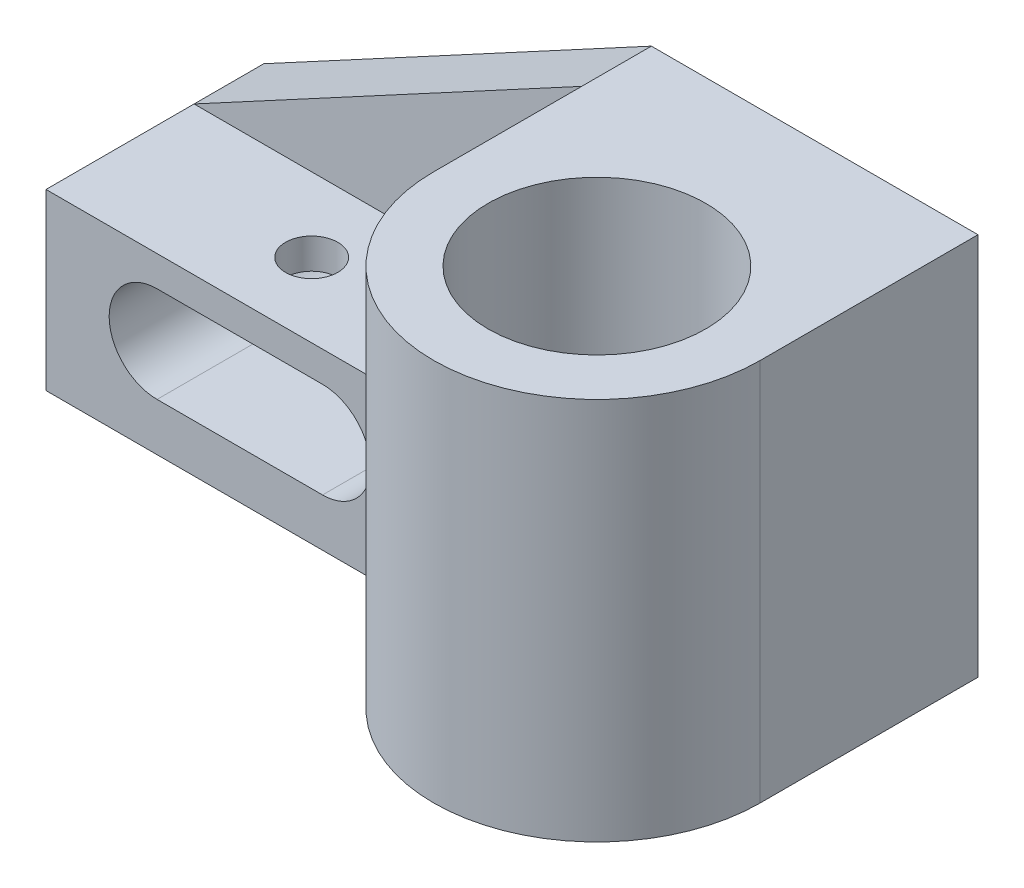
ISO-10303-21;
HEADER;
FILE_DESCRIPTION(('STEP AP214'),'2;1');
FILE_NAME('part.step','',(''),(''),'','','');
FILE_SCHEMA(('AUTOMOTIVE_DESIGN { 1 0 10303 214 1 1 1 1 }'));
ENDSEC;
DATA;
#1=APPLICATION_CONTEXT('core data for automotive mechanical design processes');
#2=APPLICATION_PROTOCOL_DEFINITION('international standard','automotive_design',2000,#1);
#3=PRODUCT_CONTEXT('',#1,'mechanical');
#4=PRODUCT('Part','Part','',(#3));
#5=PRODUCT_RELATED_PRODUCT_CATEGORY('part','',(#4));
#6=PRODUCT_DEFINITION_FORMATION('','',#4);
#7=PRODUCT_DEFINITION_CONTEXT('part definition',#1,'design');
#8=PRODUCT_DEFINITION('design','',#6,#7);
#9=PRODUCT_DEFINITION_SHAPE('','',#8);
#10=(LENGTH_UNIT() NAMED_UNIT(*) SI_UNIT(.MILLI.,.METRE.));
#11=(NAMED_UNIT(*) PLANE_ANGLE_UNIT() SI_UNIT($,.RADIAN.));
#12=(NAMED_UNIT(*) SI_UNIT($,.STERADIAN.) SOLID_ANGLE_UNIT());
#13=UNCERTAINTY_MEASURE_WITH_UNIT(LENGTH_MEASURE(1.E-05),#10,'distance_accuracy_value','');
#14=(GEOMETRIC_REPRESENTATION_CONTEXT(3) GLOBAL_UNCERTAINTY_ASSIGNED_CONTEXT((#13)) GLOBAL_UNIT_ASSIGNED_CONTEXT((#10,
#11,#12)) REPRESENTATION_CONTEXT('',''));
#15=CARTESIAN_POINT('',(0.,0.,0.));
#16=DIRECTION('',(0.,0.,1.));
#17=DIRECTION('',(1.,0.,0.));
#18=AXIS2_PLACEMENT_3D('',#15,#16,#17);
#19=CARTESIAN_POINT('',(89.,44.,50.));
#20=DIRECTION('',(1.,0.,0.));
#21=DIRECTION('',(0.,0.,-1.));
#22=AXIS2_PLACEMENT_3D('',#19,#20,#21);
#23=PLANE('',#22);
#24=DIRECTION('',(0.,0.,1.));
#25=VECTOR('',#24,1.);
#26=CARTESIAN_POINT('',(89.,48.,50.));
#27=LINE('',#26,#25);
#28=CARTESIAN_POINT('',(89.,48.,16.));
#29=VERTEX_POINT('',#28);
#30=CARTESIAN_POINT('',(89.,48.,50.));
#31=VERTEX_POINT('',#30);
#32=EDGE_CURVE('E179',#29,#31,#27,.T.);
#33=ORIENTED_EDGE('',*,*,#32,.F.);
#34=DIRECTION('',(0.,-1.,0.));
#35=VECTOR('',#34,1.);
#36=CARTESIAN_POINT('',(89.,44.,16.));
#37=LINE('',#36,#35);
#38=CARTESIAN_POINT('',(89.,0.,16.));
#39=VERTEX_POINT('',#38);
#40=EDGE_CURVE('E197',#29,#39,#37,.T.);
#41=ORIENTED_EDGE('',*,*,#40,.T.);
#42=DIRECTION('',(0.,0.,1.));
#43=VECTOR('',#42,1.);
#44=CARTESIAN_POINT('',(89.,0.,50.));
#45=LINE('',#44,#43);
#46=CARTESIAN_POINT('',(89.,0.,50.));
#47=VERTEX_POINT('',#46);
#48=EDGE_CURVE('E207',#39,#47,#45,.T.);
#49=ORIENTED_EDGE('',*,*,#48,.T.);
#50=DIRECTION('',(0.,-1.,0.));
#51=VECTOR('',#50,1.);
#52=CARTESIAN_POINT('',(89.,44.,50.));
#53=LINE('',#52,#51);
#54=EDGE_CURVE('E206',#31,#47,#53,.T.);
#55=ORIENTED_EDGE('',*,*,#54,.F.);
#56=EDGE_LOOP('',(#33,#41,#49,#55));
#57=FACE_BOUND('',#56,.T.);
#58=ADVANCED_FACE('F44',(#57),#23,.F.);
#59=CARTESIAN_POINT('',(0.,0.,0.));
#60=DIRECTION('',(0.,0.,1.));
#61=DIRECTION('',(1.,0.,0.));
#62=AXIS2_PLACEMENT_3D('',#59,#60,#61);
#63=PLANE('',#62);
#64=CARTESIAN_POINT('',(25.5,-18.,0.));
#65=DIRECTION('',(0.,0.,1.));
#66=DIRECTION('',(1.,0.,0.));
#67=AXIS2_PLACEMENT_3D('',#64,#65,#66);
#68=CIRCLE('',#67,11.);
#69=CARTESIAN_POINT('',(25.5,-7.,0.));
#70=VERTEX_POINT('',#69);
#71=CARTESIAN_POINT('',(25.5,-29.,0.));
#72=VERTEX_POINT('',#71);
#73=EDGE_CURVE('E138',#70,#72,#68,.T.);
#74=ORIENTED_EDGE('',*,*,#73,.T.);
#75=DIRECTION('',(1.,0.,0.));
#76=VECTOR('',#75,1.);
#77=CARTESIAN_POINT('',(0.,-29.,0.));
#78=LINE('',#77,#76);
#79=CARTESIAN_POINT('',(63.5,-29.,0.));
#80=VERTEX_POINT('',#79);
#81=EDGE_CURVE('E134',#72,#80,#78,.T.);
#82=ORIENTED_EDGE('',*,*,#81,.T.);
#83=CARTESIAN_POINT('',(63.5,-18.,0.));
#84=DIRECTION('',(0.,0.,1.));
#85=DIRECTION('',(1.,0.,0.));
#86=AXIS2_PLACEMENT_3D('',#83,#84,#85);
#87=CIRCLE('',#86,11.);
#88=CARTESIAN_POINT('',(63.5,-7.00000000000001,0.));
#89=VERTEX_POINT('',#88);
#90=EDGE_CURVE('E142',#80,#89,#87,.T.);
#91=ORIENTED_EDGE('',*,*,#90,.T.);
#92=DIRECTION('',(1.,0.,0.));
#93=VECTOR('',#92,1.);
#94=CARTESIAN_POINT('',(0.,-6.99999999999999,0.));
#95=LINE('',#94,#93);
#96=EDGE_CURVE('E143',#70,#89,#95,.T.);
#97=ORIENTED_EDGE('',*,*,#96,.F.);
#98=EDGE_LOOP('',(#74,#82,#91,#97));
#99=FACE_BOUND('',#98,.T.);
#100=DIRECTION('',(0.,1.,0.));
#101=VECTOR('',#100,1.);
#102=CARTESIAN_POINT('',(164.,-44.,0.));
#103=LINE('',#102,#101);
#104=CARTESIAN_POINT('',(164.,-40.,0.));
#105=VERTEX_POINT('',#104);
#106=CARTESIAN_POINT('',(164.,48.,0.));
#107=VERTEX_POINT('',#106);
#108=EDGE_CURVE('E211',#105,#107,#103,.T.);
#109=ORIENTED_EDGE('',*,*,#108,.F.);
#110=DIRECTION('',(1.,0.,0.));
#111=VECTOR('',#110,1.);
#112=CARTESIAN_POINT('',(0.,-40.,0.));
#113=LINE('',#112,#111);
#114=CARTESIAN_POINT('',(0.,-40.,0.));
#115=VERTEX_POINT('',#114);
#116=EDGE_CURVE('E219',#115,#105,#113,.T.);
#117=ORIENTED_EDGE('',*,*,#116,.F.);
#118=DIRECTION('',(0.,-1.,0.));
#119=VECTOR('',#118,1.);
#120=CARTESIAN_POINT('',(0.,0.,0.));
#121=LINE('',#120,#119);
#122=CARTESIAN_POINT('',(0.,0.,0.));
#123=VERTEX_POINT('',#122);
#124=EDGE_CURVE('E213',#123,#115,#121,.T.);
#125=ORIENTED_EDGE('',*,*,#124,.F.);
#126=DIRECTION('',(0.880153354052785,0.474689449376783,0.));
#127=VECTOR('',#126,1.);
#128=CARTESIAN_POINT('',(0.,0.,0.));
#129=LINE('',#128,#127);
#130=CARTESIAN_POINT('',(89.,48.,0.));
#131=VERTEX_POINT('',#130);
#132=EDGE_CURVE('E172',#123,#131,#129,.T.);
#133=ORIENTED_EDGE('',*,*,#132,.T.);
#134=DIRECTION('',(-1.,0.,0.));
#135=VECTOR('',#134,1.);
#136=CARTESIAN_POINT('',(89.,48.,0.));
#137=LINE('',#136,#135);
#138=EDGE_CURVE('E191',#107,#131,#137,.T.);
#139=ORIENTED_EDGE('',*,*,#138,.F.);
#140=EDGE_LOOP('',(#109,#117,#125,#133,#139));
#141=FACE_BOUND('',#140,.T.);
#142=ADVANCED_FACE('F146',(#99,#141),#63,.F.);
#143=CARTESIAN_POINT('',(164.,-44.,16.));
#144=DIRECTION('',(1.,0.,0.));
#145=DIRECTION('',(0.,0.,-1.));
#146=AXIS2_PLACEMENT_3D('',#143,#144,#145);
#147=PLANE('',#146);
#148=DIRECTION('',(0.,1.,0.));
#149=VECTOR('',#148,1.);
#150=CARTESIAN_POINT('',(164.,-44.,50.));
#151=LINE('',#150,#149);
#152=CARTESIAN_POINT('',(164.,-40.,50.));
#153=VERTEX_POINT('',#152);
#154=CARTESIAN_POINT('',(164.,48.,50.));
#155=VERTEX_POINT('',#154);
#156=EDGE_CURVE('E214',#153,#155,#151,.T.);
#157=ORIENTED_EDGE('',*,*,#156,.F.);
#158=DIRECTION('',(0.,0.,1.));
#159=VECTOR('',#158,1.);
#160=CARTESIAN_POINT('',(164.,-40.,50.));
#161=LINE('',#160,#159);
#162=EDGE_CURVE('E192',#105,#153,#161,.T.);
#163=ORIENTED_EDGE('',*,*,#162,.F.);
#164=ORIENTED_EDGE('',*,*,#108,.T.);
#165=DIRECTION('',(0.,0.,-1.));
#166=VECTOR('',#165,1.);
#167=CARTESIAN_POINT('',(164.,48.,0.));
#168=LINE('',#167,#166);
#169=EDGE_CURVE('E186',#155,#107,#168,.T.);
#170=ORIENTED_EDGE('',*,*,#169,.F.);
#171=EDGE_LOOP('',(#157,#163,#164,#170));
#172=FACE_BOUND('',#171,.T.);
#173=ADVANCED_FACE('F256',(#172),#147,.T.);
#174=CARTESIAN_POINT('',(126.5,-44.,50.));
#175=DIRECTION('',(0.,1.,0.));
#176=DIRECTION('',(0.,0.,1.));
#177=AXIS2_PLACEMENT_3D('',#174,#175,#176);
#178=CYLINDRICAL_SURFACE('',#177,37.5);
#179=DIRECTION('',(0.,1.,0.));
#180=VECTOR('',#179,1.);
#181=CARTESIAN_POINT('',(89.,-40.,50.));
#182=LINE('',#181,#180);
#183=CARTESIAN_POINT('',(89.,-40.,50.));
#184=VERTEX_POINT('',#183);
#185=EDGE_CURVE('E224',#184,#47,#182,.T.);
#186=ORIENTED_EDGE('',*,*,#185,.F.);
#187=CARTESIAN_POINT('',(126.5,-40.,50.));
#188=DIRECTION('',(0.,-1.,0.));
#189=DIRECTION('',(0.,0.,-1.));
#190=AXIS2_PLACEMENT_3D('',#187,#188,#189);
#191=CIRCLE('',#190,37.5);
#192=EDGE_CURVE('E200',#153,#184,#191,.T.);
#193=ORIENTED_EDGE('',*,*,#192,.F.);
#194=ORIENTED_EDGE('',*,*,#156,.T.);
#195=CARTESIAN_POINT('',(126.5,48.,50.));
#196=DIRECTION('',(0.,1.,0.));
#197=DIRECTION('',(0.,0.,1.));
#198=AXIS2_PLACEMENT_3D('',#195,#196,#197);
#199=CIRCLE('',#198,37.5);
#200=EDGE_CURVE('E187',#31,#155,#199,.T.);
#201=ORIENTED_EDGE('',*,*,#200,.F.);
#202=ORIENTED_EDGE('',*,*,#54,.T.);
#203=EDGE_LOOP('',(#186,#193,#194,#201,#202));
#204=FACE_BOUND('',#203,.T.);
#205=ADVANCED_FACE('F249',(#204),#178,.T.);
#206=CARTESIAN_POINT('',(89.,0.,50.));
#207=DIRECTION('',(0.,-1.,0.));
#208=DIRECTION('',(0.,0.,-1.));
#209=AXIS2_PLACEMENT_3D('',#206,#207,#208);
#210=PLANE('',#209);
#211=CARTESIAN_POINT('',(44.,0.,33.));
#212=DIRECTION('',(0.,1.,0.));
#213=DIRECTION('',(0.,0.,1.));
#214=AXIS2_PLACEMENT_3D('',#211,#212,#213);
#215=CIRCLE('',#214,5.99999999999999);
#216=CARTESIAN_POINT('',(44.,0.,39.));
#217=VERTEX_POINT('',#216);
#218=EDGE_CURVE('E156',#217,#217,#215,.T.);
#219=ORIENTED_EDGE('',*,*,#218,.F.);
#220=EDGE_LOOP('',(#219));
#221=FACE_BOUND('',#220,.T.);
#222=DIRECTION('',(-1.,0.,0.));
#223=VECTOR('',#222,1.);
#224=CARTESIAN_POINT('',(89.,0.,16.));
#225=LINE('',#224,#223);
#226=CARTESIAN_POINT('',(0.,0.,16.));
#227=VERTEX_POINT('',#226);
#228=EDGE_CURVE('E199',#39,#227,#225,.T.);
#229=ORIENTED_EDGE('',*,*,#228,.T.);
#230=DIRECTION('',(0.,0.,-1.));
#231=VECTOR('',#230,1.);
#232=CARTESIAN_POINT('',(0.,0.,50.));
#233=LINE('',#232,#231);
#234=CARTESIAN_POINT('',(0.,0.,50.));
#235=VERTEX_POINT('',#234);
#236=EDGE_CURVE('E11',#235,#227,#233,.T.);
#237=ORIENTED_EDGE('',*,*,#236,.F.);
#238=DIRECTION('',(-1.,0.,0.));
#239=VECTOR('',#238,1.);
#240=CARTESIAN_POINT('',(89.,0.,50.));
#241=LINE('',#240,#239);
#242=EDGE_CURVE('E216',#47,#235,#241,.T.);
#243=ORIENTED_EDGE('',*,*,#242,.F.);
#244=ORIENTED_EDGE('',*,*,#48,.F.);
#245=EDGE_LOOP('',(#229,#237,#243,#244));
#246=FACE_BOUND('',#245,.T.);
#247=ADVANCED_FACE('F50',(#221,#246),#210,.F.);
#248=CARTESIAN_POINT('',(0.,0.,50.));
#249=DIRECTION('',(1.,0.,0.));
#250=DIRECTION('',(0.,0.,-1.));
#251=AXIS2_PLACEMENT_3D('',#248,#249,#250);
#252=PLANE('',#251);
#253=ORIENTED_EDGE('',*,*,#124,.T.);
#254=DIRECTION('',(0.,0.,-1.));
#255=VECTOR('',#254,1.);
#256=CARTESIAN_POINT('',(0.,-40.,50.));
#257=LINE('',#256,#255);
#258=CARTESIAN_POINT('',(0.,-40.,50.));
#259=VERTEX_POINT('',#258);
#260=EDGE_CURVE('E53',#259,#115,#257,.T.);
#261=ORIENTED_EDGE('',*,*,#260,.F.);
#262=DIRECTION('',(0.,-1.,0.));
#263=VECTOR('',#262,1.);
#264=CARTESIAN_POINT('',(0.,0.,50.));
#265=LINE('',#264,#263);
#266=EDGE_CURVE('E217',#235,#259,#265,.T.);
#267=ORIENTED_EDGE('',*,*,#266,.F.);
#268=ORIENTED_EDGE('',*,*,#236,.T.);
#269=DIRECTION('',(0.,0.,-1.));
#270=VECTOR('',#269,1.);
#271=CARTESIAN_POINT('',(0.,0.,16.));
#272=LINE('',#271,#270);
#273=EDGE_CURVE('E203',#227,#123,#272,.T.);
#274=ORIENTED_EDGE('',*,*,#273,.T.);
#275=EDGE_LOOP('',(#253,#261,#267,#268,#274));
#276=FACE_BOUND('',#275,.T.);
#277=ADVANCED_FACE('F289',(#276),#252,.F.);
#278=CARTESIAN_POINT('',(0.,-40.,50.));
#279=DIRECTION('',(0.,1.,0.));
#280=DIRECTION('',(0.,0.,1.));
#281=AXIS2_PLACEMENT_3D('',#278,#279,#280);
#282=PLANE('',#281);
#283=CARTESIAN_POINT('',(126.5,-40.,50.));
#284=DIRECTION('',(0.,1.,0.));
#285=DIRECTION('',(0.,0.,1.));
#286=AXIS2_PLACEMENT_3D('',#283,#284,#285);
#287=CIRCLE('',#286,25.);
#288=CARTESIAN_POINT('',(126.5,-40.,75.));
#289=VERTEX_POINT('',#288);
#290=EDGE_CURVE('E171',#289,#289,#287,.T.);
#291=ORIENTED_EDGE('',*,*,#290,.T.);
#292=EDGE_LOOP('',(#291));
#293=FACE_BOUND('',#292,.T.);
#294=ORIENTED_EDGE('',*,*,#116,.T.);
#295=ORIENTED_EDGE('',*,*,#162,.T.);
#296=ORIENTED_EDGE('',*,*,#192,.T.);
#297=DIRECTION('',(1.,0.,0.));
#298=VECTOR('',#297,1.);
#299=CARTESIAN_POINT('',(0.,-40.,50.));
#300=LINE('',#299,#298);
#301=EDGE_CURVE('E225',#259,#184,#300,.T.);
#302=ORIENTED_EDGE('',*,*,#301,.F.);
#303=ORIENTED_EDGE('',*,*,#260,.T.);
#304=EDGE_LOOP('',(#294,#295,#296,#302,#303));
#305=FACE_BOUND('',#304,.T.);
#306=ADVANCED_FACE('F273',(#293,#305),#282,.F.);
#307=CARTESIAN_POINT('',(0.,0.,50.));
#308=DIRECTION('',(0.,0.,1.));
#309=DIRECTION('',(1.,0.,0.));
#310=AXIS2_PLACEMENT_3D('',#307,#308,#309);
#311=PLANE('',#310);
#312=DIRECTION('',(1.,0.,0.));
#313=VECTOR('',#312,1.);
#314=CARTESIAN_POINT('',(0.,-29.,50.));
#315=LINE('',#314,#313);
#316=CARTESIAN_POINT('',(25.5,-29.,50.));
#317=VERTEX_POINT('',#316);
#318=CARTESIAN_POINT('',(63.5,-29.,50.));
#319=VERTEX_POINT('',#318);
#320=EDGE_CURVE('E69',#317,#319,#315,.T.);
#321=ORIENTED_EDGE('',*,*,#320,.F.);
#322=CARTESIAN_POINT('',(25.5,-18.,50.));
#323=DIRECTION('',(0.,0.,1.));
#324=DIRECTION('',(1.,0.,0.));
#325=AXIS2_PLACEMENT_3D('',#322,#323,#324);
#326=CIRCLE('',#325,11.);
#327=CARTESIAN_POINT('',(25.5,-7.,50.));
#328=VERTEX_POINT('',#327);
#329=EDGE_CURVE('E147',#328,#317,#326,.T.);
#330=ORIENTED_EDGE('',*,*,#329,.F.);
#331=DIRECTION('',(1.,0.,0.));
#332=VECTOR('',#331,1.);
#333=CARTESIAN_POINT('',(0.,-6.99999999999999,50.));
#334=LINE('',#333,#332);
#335=CARTESIAN_POINT('',(63.5,-7.00000000000001,50.));
#336=VERTEX_POINT('',#335);
#337=EDGE_CURVE('E153',#328,#336,#334,.T.);
#338=ORIENTED_EDGE('',*,*,#337,.T.);
#339=CARTESIAN_POINT('',(63.5,-18.,50.));
#340=DIRECTION('',(0.,0.,1.));
#341=DIRECTION('',(1.,0.,0.));
#342=AXIS2_PLACEMENT_3D('',#339,#340,#341);
#343=CIRCLE('',#342,11.);
#344=EDGE_CURVE('E163',#319,#336,#343,.T.);
#345=ORIENTED_EDGE('',*,*,#344,.F.);
#346=EDGE_LOOP('',(#321,#330,#338,#345));
#347=FACE_BOUND('',#346,.T.);
#348=ORIENTED_EDGE('',*,*,#242,.T.);
#349=ORIENTED_EDGE('',*,*,#266,.T.);
#350=ORIENTED_EDGE('',*,*,#301,.T.);
#351=ORIENTED_EDGE('',*,*,#185,.T.);
#352=EDGE_LOOP('',(#348,#349,#350,#351));
#353=FACE_BOUND('',#352,.T.);
#354=ADVANCED_FACE('F244',(#347,#353),#311,.T.);
#355=CARTESIAN_POINT('',(0.,0.,16.));
#356=DIRECTION('',(0.,0.,-1.));
#357=DIRECTION('',(-1.,0.,0.));
#358=AXIS2_PLACEMENT_3D('',#355,#356,#357);
#359=PLANE('',#358);
#360=ORIENTED_EDGE('',*,*,#40,.F.);
#361=DIRECTION('',(0.880153354052785,0.474689449376783,0.));
#362=VECTOR('',#361,1.);
#363=CARTESIAN_POINT('',(0.,0.,16.));
#364=LINE('',#363,#362);
#365=EDGE_CURVE('E180',#227,#29,#364,.T.);
#366=ORIENTED_EDGE('',*,*,#365,.F.);
#367=ORIENTED_EDGE('',*,*,#228,.F.);
#368=EDGE_LOOP('',(#360,#366,#367));
#369=FACE_BOUND('',#368,.T.);
#370=ADVANCED_FACE('F262',(#369),#359,.F.);
#371=CARTESIAN_POINT('',(126.5,48.,50.));
#372=DIRECTION('',(0.,1.,0.));
#373=DIRECTION('',(0.,0.,1.));
#374=AXIS2_PLACEMENT_3D('',#371,#372,#373);
#375=PLANE('',#374);
#376=CARTESIAN_POINT('',(126.5,48.,50.));
#377=DIRECTION('',(0.,1.,0.));
#378=DIRECTION('',(0.,0.,1.));
#379=AXIS2_PLACEMENT_3D('',#376,#377,#378);
#380=CIRCLE('',#379,25.);
#381=CARTESIAN_POINT('',(126.5,48.,75.));
#382=VERTEX_POINT('',#381);
#383=EDGE_CURVE('E170',#382,#382,#380,.T.);
#384=ORIENTED_EDGE('',*,*,#383,.F.);
#385=EDGE_LOOP('',(#384));
#386=FACE_BOUND('',#385,.T.);
#387=EDGE_CURVE('E182',#131,#29,#27,.T.);
#388=ORIENTED_EDGE('',*,*,#387,.T.);
#389=ORIENTED_EDGE('',*,*,#32,.T.);
#390=ORIENTED_EDGE('',*,*,#200,.T.);
#391=ORIENTED_EDGE('',*,*,#169,.T.);
#392=ORIENTED_EDGE('',*,*,#138,.T.);
#393=EDGE_LOOP('',(#388,#389,#390,#391,#392));
#394=FACE_BOUND('',#393,.T.);
#395=ADVANCED_FACE('F251',(#386,#394),#375,.T.);
#396=CARTESIAN_POINT('',(0.,0.,16.));
#397=DIRECTION('',(-0.474689449376783,0.880153354052785,0.));
#398=DIRECTION('',(-0.880153354052785,-0.474689449376783,0.));
#399=AXIS2_PLACEMENT_3D('',#396,#397,#398);
#400=PLANE('',#399);
#401=ORIENTED_EDGE('',*,*,#132,.F.);
#402=ORIENTED_EDGE('',*,*,#273,.F.);
#403=ORIENTED_EDGE('',*,*,#365,.T.);
#404=ORIENTED_EDGE('',*,*,#387,.F.);
#405=EDGE_LOOP('',(#401,#402,#403,#404));
#406=FACE_BOUND('',#405,.T.);
#407=ADVANCED_FACE('F263',(#406),#400,.T.);
#408=CARTESIAN_POINT('',(126.5,-40.,50.));
#409=DIRECTION('',(0.,1.,0.));
#410=DIRECTION('',(0.,0.,1.));
#411=AXIS2_PLACEMENT_3D('',#408,#409,#410);
#412=CYLINDRICAL_SURFACE('',#411,25.);
#413=ORIENTED_EDGE('',*,*,#290,.F.);
#414=EDGE_LOOP('',(#413));
#415=FACE_BOUND('',#414,.T.);
#416=ORIENTED_EDGE('',*,*,#383,.T.);
#417=EDGE_LOOP('',(#416));
#418=FACE_BOUND('',#417,.T.);
#419=ADVANCED_FACE('F322',(#415,#418),#412,.F.);
#420=CARTESIAN_POINT('',(0.,-29.,0.));
#421=DIRECTION('',(0.,-1.,0.));
#422=DIRECTION('',(1.,0.,0.));
#423=AXIS2_PLACEMENT_3D('',#420,#421,#422);
#424=PLANE('',#423);
#425=ORIENTED_EDGE('',*,*,#320,.T.);
#426=DIRECTION('',(0.,0.,1.));
#427=VECTOR('',#426,1.);
#428=CARTESIAN_POINT('',(63.5,-29.,0.));
#429=LINE('',#428,#427);
#430=EDGE_CURVE('E135',#80,#319,#429,.T.);
#431=ORIENTED_EDGE('',*,*,#430,.F.);
#432=ORIENTED_EDGE('',*,*,#81,.F.);
#433=DIRECTION('',(0.,0.,1.));
#434=VECTOR('',#433,1.);
#435=CARTESIAN_POINT('',(25.5,-29.,0.));
#436=LINE('',#435,#434);
#437=EDGE_CURVE('E164',#72,#317,#436,.T.);
#438=ORIENTED_EDGE('',*,*,#437,.T.);
#439=EDGE_LOOP('',(#425,#431,#432,#438));
#440=FACE_BOUND('',#439,.T.);
#441=ADVANCED_FACE('F133',(#440),#424,.F.);
#442=CARTESIAN_POINT('',(25.5,-18.,0.));
#443=DIRECTION('',(0.,0.,1.));
#444=DIRECTION('',(1.,0.,0.));
#445=AXIS2_PLACEMENT_3D('',#442,#443,#444);
#446=CYLINDRICAL_SURFACE('',#445,11.);
#447=ORIENTED_EDGE('',*,*,#329,.T.);
#448=ORIENTED_EDGE('',*,*,#437,.F.);
#449=ORIENTED_EDGE('',*,*,#73,.F.);
#450=DIRECTION('',(0.,0.,1.));
#451=VECTOR('',#450,1.);
#452=CARTESIAN_POINT('',(25.5,-7.,0.));
#453=LINE('',#452,#451);
#454=EDGE_CURVE('E166',#70,#328,#453,.T.);
#455=ORIENTED_EDGE('',*,*,#454,.T.);
#456=EDGE_LOOP('',(#447,#448,#449,#455));
#457=FACE_BOUND('',#456,.T.);
#458=ADVANCED_FACE('F314',(#457),#446,.F.);
#459=CARTESIAN_POINT('',(0.,-6.99999999999999,0.));
#460=DIRECTION('',(0.,-1.,0.));
#461=DIRECTION('',(1.,0.,0.));
#462=AXIS2_PLACEMENT_3D('',#459,#460,#461);
#463=PLANE('',#462);
#464=CARTESIAN_POINT('',(44.,-7.,33.));
#465=DIRECTION('',(0.,-1.,0.));
#466=DIRECTION('',(1.,0.,0.));
#467=AXIS2_PLACEMENT_3D('',#464,#465,#466);
#468=CIRCLE('',#467,5.99999999999999);
#469=CARTESIAN_POINT('',(50.,-7.00000000000001,33.));
#470=VERTEX_POINT('',#469);
#471=EDGE_CURVE('E47',#470,#470,#468,.T.);
#472=ORIENTED_EDGE('',*,*,#471,.F.);
#473=EDGE_LOOP('',(#472));
#474=FACE_BOUND('',#473,.T.);
#475=ORIENTED_EDGE('',*,*,#337,.F.);
#476=ORIENTED_EDGE('',*,*,#454,.F.);
#477=ORIENTED_EDGE('',*,*,#96,.T.);
#478=DIRECTION('',(0.,0.,1.));
#479=VECTOR('',#478,1.);
#480=CARTESIAN_POINT('',(63.5,-7.00000000000001,0.));
#481=LINE('',#480,#479);
#482=EDGE_CURVE('E61',#89,#336,#481,.T.);
#483=ORIENTED_EDGE('',*,*,#482,.T.);
#484=EDGE_LOOP('',(#475,#476,#477,#483));
#485=FACE_BOUND('',#484,.T.);
#486=ADVANCED_FACE('F315',(#474,#485),#463,.T.);
#487=CARTESIAN_POINT('',(63.5,-18.,0.));
#488=DIRECTION('',(0.,0.,1.));
#489=DIRECTION('',(1.,0.,0.));
#490=AXIS2_PLACEMENT_3D('',#487,#488,#489);
#491=CYLINDRICAL_SURFACE('',#490,11.);
#492=ORIENTED_EDGE('',*,*,#344,.T.);
#493=ORIENTED_EDGE('',*,*,#482,.F.);
#494=ORIENTED_EDGE('',*,*,#90,.F.);
#495=ORIENTED_EDGE('',*,*,#430,.T.);
#496=EDGE_LOOP('',(#492,#493,#494,#495));
#497=FACE_BOUND('',#496,.T.);
#498=ADVANCED_FACE('F145',(#497),#491,.F.);
#499=CARTESIAN_POINT('',(44.,-10.,33.));
#500=DIRECTION('',(0.,1.,0.));
#501=DIRECTION('',(0.,0.,1.));
#502=AXIS2_PLACEMENT_3D('',#499,#500,#501);
#503=CYLINDRICAL_SURFACE('',#502,5.99999999999999);
#504=ORIENTED_EDGE('',*,*,#471,.T.);
#505=EDGE_LOOP('',(#504));
#506=FACE_BOUND('',#505,.T.);
#507=ORIENTED_EDGE('',*,*,#218,.T.);
#508=EDGE_LOOP('',(#507));
#509=FACE_BOUND('',#508,.T.);
#510=ADVANCED_FACE('F309',(#506,#509),#503,.F.);
#511=CLOSED_SHELL('',(#58,#142,#173,#205,#247,#277,#306,#354,#370,#395,#407,#419,#441,#458,#486,
#498,#510));
#512=MANIFOLD_SOLID_BREP('B2',#511);
#513=ADVANCED_BREP_SHAPE_REPRESENTATION('',(#18,#512),#14);
#514=SHAPE_DEFINITION_REPRESENTATION(#9,#513);
ENDSEC;
END-ISO-10303-21;
